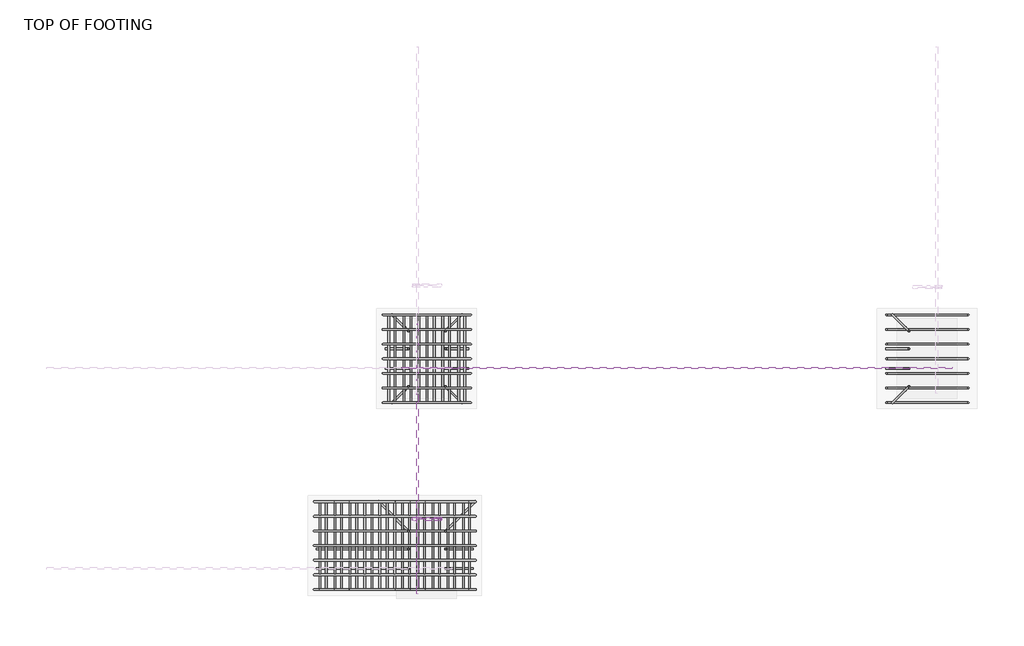
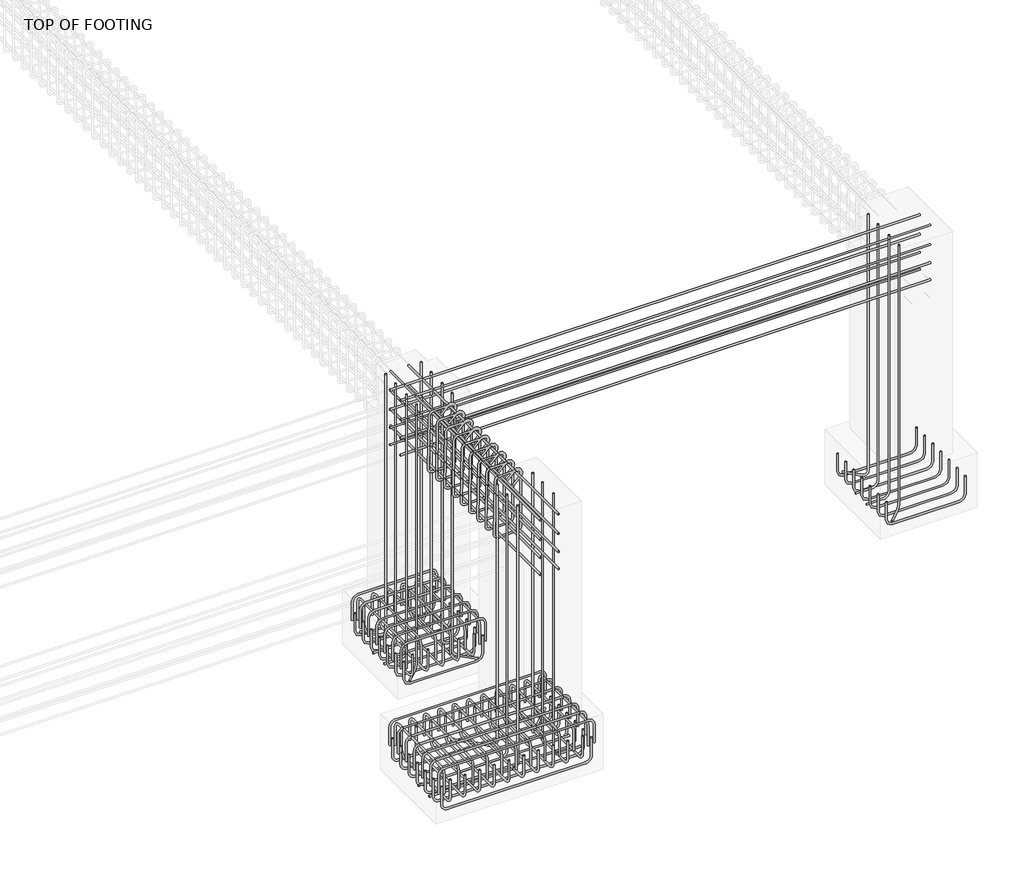
# One storey, part 3 of 8: 31 reinforcing bars.
"""IFC4 building model written with IfcOpenShell, lengths in millimetres."""

from ifc_helpers import new_model, si_unit, point, frame, origin, place, context, project, spatial, polyline, circle_curve, trimmed, segment, composite_curve, source, transform, mapped, element, save
from ifc_brep_helpers import swept_disk

model = new_model("IFC4")

# Units and contexts
model_context = context("Model", 3, world=origin())
ifc_project = project(units=[si_unit("LENGTHUNIT", "METRE", prefix="MILLI")], contexts=[model_context])

# Site, building, storey
site = spatial("IfcSite", under=ifc_project)
building = spatial("IfcBuilding", under=site)
storey = spatial("IfcBuildingStorey", under=building, Name="TOP OF FOOTING", Elevation=-1828.8)

# Reinforcing bars
placement = place(None, origin())
reinforcing_bar_shape = source(origin(), model_context, "Body", "SolidModel", [
    swept_disk(composite_curve([segment(polyline([(2354.4122182, -154.3579757, -2021.245224), (2354.4122182, -154.3579757, -2168.545224)]), True, "CONTINUOUS"), segment(trimmed(circle_curve(frame((2308.0622182, -154.3579757, -2168.545224), z_axis=(0.0, 1.0, 0.0), x_axis=(46.34999999999991, 0.0, 0.0)), 46.35), [point((2354.4122182, -154.3579757, -2168.545224))], [point((2308.0622182, -154.3579757, -2214.895224))], True, "CARTESIAN"), True, "CONTINUOUS"), segment(polyline([(2308.0622182, -154.3579757, -2214.895224), (1787.1241353, -154.3579757, -2214.895224)]), True, "CONTINUOUS"), segment(trimmed(circle_curve(frame((1787.1241353, -154.3579757, -2168.545224), z_axis=(0.0, 1.0, 0.0), x_axis=(0.0, 0.0, -46.34999999999991)), 46.35), [point((1787.1241353, -154.3579757, -2214.895224))], [point((1740.7741353, -154.3579757, -2168.545224))], True, "CARTESIAN"), True, "CONTINUOUS"), segment(polyline([(1740.7741353, -154.3579757, -2168.545224), (1740.7741353, -154.3579757, -2021.245224)]), True, "CONTINUOUS")], self_intersect=False), 6.35),
])
element("IfcReinforcingBar", 1, at=placement, inside=storey, context=model_context, shape_type="MappedRepresentation", body=[
    mapped(reinforcing_bar_shape, transform((0.0, 0.0, 0.0), x_axis=(1.0, 0.0, 0.0), y_axis=(0.0, 1.0, 0.0), z_axis=(0.0, 0.0, 1.0))),
    mapped(reinforcing_bar_shape, transform((0.0, -109.55, 0.0), x_axis=(1.0, 0.0, 0.0), y_axis=(0.0, 1.0, 0.0), z_axis=(0.0, 0.0, 1.0))),
    mapped(reinforcing_bar_shape, transform((0.0, -219.1, 0.0), x_axis=(1.0, 0.0, 0.0), y_axis=(0.0, 1.0, 0.0), z_axis=(0.0, 0.0, 1.0))),
    mapped(reinforcing_bar_shape, transform((0.0, -328.65, 0.0), x_axis=(1.0, 0.0, 0.0), y_axis=(0.0, 1.0, 0.0), z_axis=(0.0, 0.0, 1.0))),
    mapped(reinforcing_bar_shape, transform((0.0, -438.2, 0.0), x_axis=(1.0, 0.0, 0.0), y_axis=(0.0, 1.0, 0.0), z_axis=(0.0, 0.0, 1.0))),
    mapped(reinforcing_bar_shape, transform((0.0, -547.75, 0.0), x_axis=(1.0, 0.0, 0.0), y_axis=(0.0, 1.0, 0.0), z_axis=(0.0, 0.0, 1.0))),
    mapped(reinforcing_bar_shape, transform((0.0, -657.3, 0.0), x_axis=(1.0, 0.0, 0.0), y_axis=(0.0, 1.0, 0.0), z_axis=(0.0, 0.0, 1.0))),
])
reinforcing_bar_2_shape = source(origin(), model_context, "Body", "SolidModel", [
    swept_disk(composite_curve([segment(polyline([(-1395.5877818, -154.3579757, -2021.245224), (-1395.5877818, -154.3579757, -2168.545224)]), True, "CONTINUOUS"), segment(trimmed(circle_curve(frame((-1441.9377818, -154.3579757, -2168.545224), z_axis=(0.0, 1.0, 0.0), x_axis=(46.350000000000136, 0.0, 0.0)), 46.35), [point((-1395.5877818, -154.3579757, -2168.545224))], [point((-1441.9377818, -154.3579757, -2214.895224))], True, "CARTESIAN"), True, "CONTINUOUS"), segment(polyline([(-1441.9377818, -154.3579757, -2214.895224), (-1962.8758647, -154.3579757, -2214.895224)]), True, "CONTINUOUS"), segment(trimmed(circle_curve(frame((-1962.8758647, -154.3579757, -2168.545224), z_axis=(0.0, 1.0, 0.0), x_axis=(0.0, 0.0, -46.34999999999991)), 46.35), [point((-1962.8758647, -154.3579757, -2214.895224))], [point((-2009.2258647, -154.3579757, -2168.545224))], True, "CARTESIAN"), True, "CONTINUOUS"), segment(polyline([(-2009.2258647, -154.3579757, -2168.545224), (-2009.2258647, -154.3579757, -2021.245224)]), True, "CONTINUOUS")], self_intersect=False), 6.35),
])
element("IfcReinforcingBar", 2, at=placement, inside=storey, context=model_context, shape_type="MappedRepresentation", body=[
    mapped(reinforcing_bar_2_shape, transform((0.0, 0.0, 0.0), x_axis=(1.0, 0.0, 0.0), y_axis=(0.0, 1.0, 0.0), z_axis=(0.0, 0.0, 1.0))),
    mapped(reinforcing_bar_2_shape, transform((0.0, -109.55, 0.0), x_axis=(1.0, 0.0, 0.0), y_axis=(0.0, 1.0, 0.0), z_axis=(0.0, 0.0, 1.0))),
    mapped(reinforcing_bar_2_shape, transform((0.0, -219.1, 0.0), x_axis=(1.0, 0.0, 0.0), y_axis=(0.0, 1.0, 0.0), z_axis=(0.0, 0.0, 1.0))),
    mapped(reinforcing_bar_2_shape, transform((0.0, -328.65, 0.0), x_axis=(1.0, 0.0, 0.0), y_axis=(0.0, 1.0, 0.0), z_axis=(0.0, 0.0, 1.0))),
    mapped(reinforcing_bar_2_shape, transform((0.0, -438.2, 0.0), x_axis=(1.0, 0.0, 0.0), y_axis=(0.0, 1.0, 0.0), z_axis=(0.0, 0.0, 1.0))),
    mapped(reinforcing_bar_2_shape, transform((0.0, -547.75, 0.0), x_axis=(1.0, 0.0, 0.0), y_axis=(0.0, 1.0, 0.0), z_axis=(0.0, 0.0, 1.0))),
    mapped(reinforcing_bar_2_shape, transform((0.0, -657.3, 0.0), x_axis=(1.0, 0.0, 0.0), y_axis=(0.0, 1.0, 0.0), z_axis=(0.0, 0.0, 1.0))),
])
reinforcing_bar_3_shape = source(origin(), model_context, "Body", "SolidModel", [
    swept_disk(composite_curve([segment(polyline([(-2031.1461367, -154.3579757, -2068.8), (-2031.1461367, -154.3579757, -1921.5)]), True, "CONTINUOUS"), segment(trimmed(circle_curve(frame((-1984.7961367, -154.3579757, -1921.5), z_axis=(0.0, 1.0, 0.0), x_axis=(-46.34999999999991, 0.0, 0.0)), 46.35), [point((-2031.1461367, -154.3579757, -1921.5))], [point((-1984.7961367, -154.3579757, -1875.15))], True, "CARTESIAN"), True, "CONTINUOUS"), segment(polyline([(-1984.7961367, -154.3579757, -1875.15), (-1420.1961367, -154.3579757, -1875.15)]), True, "CONTINUOUS"), segment(trimmed(circle_curve(frame((-1420.1961367, -154.3579757, -1921.5), z_axis=(0.0, 1.0, 0.0), x_axis=(0.0, 0.0, 46.34999999999991)), 46.35), [point((-1420.1961367, -154.3579757, -1875.15))], [point((-1373.8461367, -154.3579757, -1921.5))], True, "CARTESIAN"), True, "CONTINUOUS"), segment(polyline([(-1373.8461367, -154.3579757, -1921.5), (-1373.8461367, -154.3579757, -2068.8)]), True, "CONTINUOUS")], self_intersect=False), 6.35),
])
element("IfcReinforcingBar", 3, at=placement, inside=storey, context=model_context, shape_type="MappedRepresentation", body=[
    mapped(reinforcing_bar_3_shape, transform((0.0, 0.0, 0.0), x_axis=(1.0, 0.0, 0.0), y_axis=(0.0, 1.0, 0.0), z_axis=(0.0, 0.0, 1.0))),
    mapped(reinforcing_bar_3_shape, transform((0.0, -109.55, 0.0), x_axis=(1.0, 0.0, 0.0), y_axis=(0.0, 1.0, 0.0), z_axis=(0.0, 0.0, 1.0))),
    mapped(reinforcing_bar_3_shape, transform((0.0, -219.1, 0.0), x_axis=(1.0, 0.0, 0.0), y_axis=(0.0, 1.0, 0.0), z_axis=(0.0, 0.0, 1.0))),
    mapped(reinforcing_bar_3_shape, transform((0.0, -328.65, 0.0), x_axis=(1.0, 0.0, 0.0), y_axis=(0.0, 1.0, 0.0), z_axis=(0.0, 0.0, 1.0))),
    mapped(reinforcing_bar_3_shape, transform((0.0, -438.2, 0.0), x_axis=(1.0, 0.0, 0.0), y_axis=(0.0, 1.0, 0.0), z_axis=(0.0, 0.0, 1.0))),
    mapped(reinforcing_bar_3_shape, transform((0.0, -547.75, 0.0), x_axis=(1.0, 0.0, 0.0), y_axis=(0.0, 1.0, 0.0), z_axis=(0.0, 0.0, 1.0))),
    mapped(reinforcing_bar_3_shape, transform((0.0, -657.3, 0.0), x_axis=(1.0, 0.0, 0.0), y_axis=(0.0, 1.0, 0.0), z_axis=(0.0, 0.0, 1.0))),
])
reinforcing_bar_4_shape = source(origin(), model_context, "Body", "SolidModel", [
    swept_disk(composite_curve([segment(polyline([(-1419.0253093, -154.3579757, -2080.9203068), (-1419.0253093, -154.3579757, -1933.6203068)]), True, "CONTINUOUS"), segment(trimmed(circle_curve(frame((-1419.0253093, -200.7079757, -1933.6203068), z_axis=(1.0, 0.0, 0.0), x_axis=(0.0, 46.349999999999994, 0.0)), 46.35), [point((-1419.0253093, -154.3579757, -1933.6203068))], [point((-1419.0253093, -200.7079757, -1887.2703068))], True, "CARTESIAN"), True, "CONTINUOUS"), segment(polyline([(-1419.0253093, -200.7079757, -1887.2703068), (-1419.0253093, -765.3079757, -1887.2703068)]), True, "CONTINUOUS"), segment(trimmed(circle_curve(frame((-1419.0253093, -765.3079757, -1933.6203068), z_axis=(1.0, 0.0, 0.0), x_axis=(0.0, 0.0, 46.34999999999991)), 46.35), [point((-1419.0253093, -765.3079757, -1887.2703068))], [point((-1419.0253093, -811.6579757, -1933.6203068))], True, "CARTESIAN"), True, "CONTINUOUS"), segment(polyline([(-1419.0253093, -811.6579757, -1933.6203068), (-1419.0253093, -811.6579757, -2080.9203068)]), True, "CONTINUOUS")], self_intersect=False), 6.35),
])
element("IfcReinforcingBar", 4, at=placement, inside=storey, context=model_context, shape_type="MappedRepresentation", body=[
    mapped(reinforcing_bar_4_shape, transform((0.0, 0.0, 0.0), x_axis=(1.0, 0.0, 0.0), y_axis=(0.0, 1.0, 0.0), z_axis=(0.0, 0.0, 1.0))),
    mapped(reinforcing_bar_4_shape, transform((-113.9683653, 0.0, 0.0), x_axis=(1.0, 0.0, 0.0), y_axis=(0.0, 1.0, 0.0), z_axis=(0.0, 0.0, 1.0))),
    mapped(reinforcing_bar_4_shape, transform((-227.9367307, 0.0, 0.0), x_axis=(1.0, 0.0, 0.0), y_axis=(0.0, 1.0, 0.0), z_axis=(0.0, 0.0, 1.0))),
    mapped(reinforcing_bar_4_shape, transform((-341.905096, 0.0, 0.0), x_axis=(1.0, 0.0, 0.0), y_axis=(0.0, 1.0, 0.0), z_axis=(0.0, 0.0, 1.0))),
    mapped(reinforcing_bar_4_shape, transform((-455.8734613, 0.0, 0.0), x_axis=(1.0, 0.0, 0.0), y_axis=(0.0, 1.0, 0.0), z_axis=(0.0, 0.0, 1.0))),
    mapped(reinforcing_bar_4_shape, transform((-569.8418267, 0.0, 0.0), x_axis=(1.0, 0.0, 0.0), y_axis=(0.0, 1.0, 0.0), z_axis=(0.0, 0.0, 1.0))),
])
reinforcing_bar_5_shape = source(origin(), model_context, "Body", "SolidModel", [
    swept_disk(composite_curve([segment(polyline([(-1941.3656272, -154.3579757, -1984.9681267), (-1941.3656272, -154.3579757, -2132.2681267)]), True, "CONTINUOUS"), segment(trimmed(circle_curve(frame((-1941.3656272, -200.7079757, -2132.2681267), z_axis=(-1.0, 0.0, 0.0), x_axis=(0.0, 46.349999999999994, 0.0)), 46.35), [point((-1941.3656272, -154.3579757, -2132.2681267))], [point((-1941.3656272, -200.7079757, -2178.6181267))], True, "CARTESIAN"), True, "CONTINUOUS"), segment(polyline([(-1941.3656272, -200.7079757, -2178.6181267), (-1941.3656272, -765.3079757, -2178.6181267)]), True, "CONTINUOUS"), segment(trimmed(circle_curve(frame((-1941.3656272, -765.3079757, -2132.2681267), z_axis=(-1.0, 0.0, 0.0), x_axis=(0.0, 0.0, -46.350000000000364)), 46.35), [point((-1941.3656272, -765.3079757, -2178.6181267))], [point((-1941.3656272, -811.6579757, -2132.2681267))], True, "CARTESIAN"), True, "CONTINUOUS"), segment(polyline([(-1941.3656272, -811.6579757, -2132.2681267), (-1941.3656272, -811.6579757, -1984.9681267)]), True, "CONTINUOUS")], self_intersect=False), 6.35),
])
element("IfcReinforcingBar", 5, at=placement, inside=storey, context=model_context, shape_type="MappedRepresentation", body=[
    mapped(reinforcing_bar_5_shape, transform((0.0, 0.0, 0.0), x_axis=(1.0, 0.0, 0.0), y_axis=(0.0, 1.0, 0.0), z_axis=(0.0, 0.0, 1.0))),
    mapped(reinforcing_bar_5_shape, transform((119.2770606, 0.0, 0.0), x_axis=(1.0, 0.0, 0.0), y_axis=(0.0, 1.0, 0.0), z_axis=(0.0, 0.0, 1.0))),
    mapped(reinforcing_bar_5_shape, transform((238.5541211, 0.0, 0.0), x_axis=(1.0, 0.0, 0.0), y_axis=(0.0, 1.0, 0.0), z_axis=(0.0, 0.0, 1.0))),
    mapped(reinforcing_bar_5_shape, transform((357.8311817, 0.0, 0.0), x_axis=(1.0, 0.0, 0.0), y_axis=(0.0, 1.0, 0.0), z_axis=(0.0, 0.0, 1.0))),
    mapped(reinforcing_bar_5_shape, transform((477.1082423, 0.0, 0.0), x_axis=(1.0, 0.0, 0.0), y_axis=(0.0, 1.0, 0.0), z_axis=(0.0, 0.0, 1.0))),
])
reinforcing_bar_6_shape = source(origin(), model_context, "Body", "SolidModel", [
    swept_disk(composite_curve([segment(polyline([(-1360.5877818, -1554.3579757, -2021.245224), (-1360.5877818, -1554.3579757, -2168.545224)]), True, "CONTINUOUS"), segment(trimmed(circle_curve(frame((-1406.9377818, -1554.3579757, -2168.545224), z_axis=(0.0, 1.0, 0.0), x_axis=(46.350000000000136, 0.0, 0.0)), 46.35), [point((-1360.5877818, -1554.3579757, -2168.545224))], [point((-1406.9377818, -1554.3579757, -2214.895224))], True, "CARTESIAN"), True, "CONTINUOUS"), segment(polyline([(-1406.9377818, -1554.3579757, -2214.895224), (-2477.8758647, -1554.3579757, -2214.895224)]), True, "CONTINUOUS"), segment(trimmed(circle_curve(frame((-2477.8758647, -1554.3579757, -2168.545224), z_axis=(0.0, 1.0, 0.0), x_axis=(0.0, 0.0, -46.34999999999991)), 46.35), [point((-2477.8758647, -1554.3579757, -2214.895224))], [point((-2524.2258647, -1554.3579757, -2168.545224))], True, "CARTESIAN"), True, "CONTINUOUS"), segment(polyline([(-2524.2258647, -1554.3579757, -2168.545224), (-2524.2258647, -1554.3579757, -2021.245224)]), True, "CONTINUOUS")], self_intersect=False), 6.35),
])
element("IfcReinforcingBar", 6, at=placement, inside=storey, context=model_context, shape_type="MappedRepresentation", body=[
    mapped(reinforcing_bar_6_shape, transform((0.0, 0.0, 0.0), x_axis=(1.0, 0.0, 0.0), y_axis=(0.0, 1.0, 0.0), z_axis=(0.0, 0.0, 1.0))),
    mapped(reinforcing_bar_6_shape, transform((0.0, -109.55, 0.0), x_axis=(1.0, 0.0, 0.0), y_axis=(0.0, 1.0, 0.0), z_axis=(0.0, 0.0, 1.0))),
    mapped(reinforcing_bar_6_shape, transform((0.0, -219.1, 0.0), x_axis=(1.0, 0.0, 0.0), y_axis=(0.0, 1.0, 0.0), z_axis=(0.0, 0.0, 1.0))),
    mapped(reinforcing_bar_6_shape, transform((0.0, -328.65, 0.0), x_axis=(1.0, 0.0, 0.0), y_axis=(0.0, 1.0, 0.0), z_axis=(0.0, 0.0, 1.0))),
    mapped(reinforcing_bar_6_shape, transform((0.0, -438.2, 0.0), x_axis=(1.0, 0.0, 0.0), y_axis=(0.0, 1.0, 0.0), z_axis=(0.0, 0.0, 1.0))),
    mapped(reinforcing_bar_6_shape, transform((0.0, -547.75, 0.0), x_axis=(1.0, 0.0, 0.0), y_axis=(0.0, 1.0, 0.0), z_axis=(0.0, 0.0, 1.0))),
    mapped(reinforcing_bar_6_shape, transform((0.0, -657.3, 0.0), x_axis=(1.0, 0.0, 0.0), y_axis=(0.0, 1.0, 0.0), z_axis=(0.0, 0.0, 1.0))),
])
reinforcing_bar_7_shape = source(origin(), model_context, "Body", "SolidModel", [
    swept_disk(composite_curve([segment(polyline([(-2546.1461367, -1554.3579757, -2068.8), (-2546.1461367, -1554.3579757, -1921.5)]), True, "CONTINUOUS"), segment(trimmed(circle_curve(frame((-2499.7961367, -1554.3579757, -1921.5), z_axis=(0.0, 1.0, 0.0), x_axis=(-46.350000000000364, 0.0, 0.0)), 46.35), [point((-2546.1461367, -1554.3579757, -1921.5))], [point((-2499.7961367, -1554.3579757, -1875.15))], True, "CARTESIAN"), True, "CONTINUOUS"), segment(polyline([(-2499.7961367, -1554.3579757, -1875.15), (-1385.1961367, -1554.3579757, -1875.15)]), True, "CONTINUOUS"), segment(trimmed(circle_curve(frame((-1385.1961367, -1554.3579757, -1921.5), z_axis=(0.0, 1.0, 0.0), x_axis=(0.0, 0.0, 46.34999999999991)), 46.35), [point((-1385.1961367, -1554.3579757, -1875.15))], [point((-1338.8461367, -1554.3579757, -1921.5))], True, "CARTESIAN"), True, "CONTINUOUS"), segment(polyline([(-1338.8461367, -1554.3579757, -1921.5), (-1338.8461367, -1554.3579757, -2068.8)]), True, "CONTINUOUS")], self_intersect=False), 6.35),
])
element("IfcReinforcingBar", 7, at=placement, inside=storey, context=model_context, shape_type="MappedRepresentation", body=[
    mapped(reinforcing_bar_7_shape, transform((0.0, 0.0, 0.0), x_axis=(1.0, 0.0, 0.0), y_axis=(0.0, 1.0, 0.0), z_axis=(0.0, 0.0, 1.0))),
    mapped(reinforcing_bar_7_shape, transform((0.0, -109.55, 0.0), x_axis=(1.0, 0.0, 0.0), y_axis=(0.0, 1.0, 0.0), z_axis=(0.0, 0.0, 1.0))),
    mapped(reinforcing_bar_7_shape, transform((0.0, -219.1, 0.0), x_axis=(1.0, 0.0, 0.0), y_axis=(0.0, 1.0, 0.0), z_axis=(0.0, 0.0, 1.0))),
    mapped(reinforcing_bar_7_shape, transform((0.0, -328.65, 0.0), x_axis=(1.0, 0.0, 0.0), y_axis=(0.0, 1.0, 0.0), z_axis=(0.0, 0.0, 1.0))),
    mapped(reinforcing_bar_7_shape, transform((0.0, -438.2, 0.0), x_axis=(1.0, 0.0, 0.0), y_axis=(0.0, 1.0, 0.0), z_axis=(0.0, 0.0, 1.0))),
    mapped(reinforcing_bar_7_shape, transform((0.0, -547.75, 0.0), x_axis=(1.0, 0.0, 0.0), y_axis=(0.0, 1.0, 0.0), z_axis=(0.0, 0.0, 1.0))),
    mapped(reinforcing_bar_7_shape, transform((0.0, -657.3, 0.0), x_axis=(1.0, 0.0, 0.0), y_axis=(0.0, 1.0, 0.0), z_axis=(0.0, 0.0, 1.0))),
])
reinforcing_bar_8_shape = source(origin(), model_context, "Body", "SolidModel", [
    swept_disk(composite_curve([segment(polyline([(-1384.0253093, -1554.3579757, -2080.9203068), (-1384.0253093, -1554.3579757, -1933.6203068)]), True, "CONTINUOUS"), segment(trimmed(circle_curve(frame((-1384.0253093, -1600.7079757, -1933.6203068), z_axis=(1.0, 0.0, 0.0), x_axis=(0.0, 46.34999999999991, 0.0)), 46.35), [point((-1384.0253093, -1554.3579757, -1933.6203068))], [point((-1384.0253093, -1600.7079757, -1887.2703068))], True, "CARTESIAN"), True, "CONTINUOUS"), segment(polyline([(-1384.0253093, -1600.7079757, -1887.2703068), (-1384.0253093, -2165.3079757, -1887.2703068)]), True, "CONTINUOUS"), segment(trimmed(circle_curve(frame((-1384.0253093, -2165.3079757, -1933.6203068), z_axis=(1.0, 0.0, 0.0), x_axis=(0.0, 0.0, 46.34999999999991)), 46.35), [point((-1384.0253093, -2165.3079757, -1887.2703068))], [point((-1384.0253093, -2211.6579757, -1933.6203068))], True, "CARTESIAN"), True, "CONTINUOUS"), segment(polyline([(-1384.0253093, -2211.6579757, -1933.6203068), (-1384.0253093, -2211.6579757, -2080.9203068)]), True, "CONTINUOUS")], self_intersect=False), 6.35),
])
element("IfcReinforcingBar", 8, at=placement, inside=storey, context=model_context, shape_type="MappedRepresentation", body=[
    mapped(reinforcing_bar_8_shape, transform((0.0, 0.0, 0.0), x_axis=(1.0, 0.0, 0.0), y_axis=(0.0, 1.0, 0.0), z_axis=(0.0, 0.0, 1.0))),
    mapped(reinforcing_bar_8_shape, transform((-111.9841827, 0.0, 0.0), x_axis=(1.0, 0.0, 0.0), y_axis=(0.0, 1.0, 0.0), z_axis=(0.0, 0.0, 1.0))),
    mapped(reinforcing_bar_8_shape, transform((-223.9683653, 0.0, 0.0), x_axis=(1.0, 0.0, 0.0), y_axis=(0.0, 1.0, 0.0), z_axis=(0.0, 0.0, 1.0))),
    mapped(reinforcing_bar_8_shape, transform((-335.952548, 0.0, 0.0), x_axis=(1.0, 0.0, 0.0), y_axis=(0.0, 1.0, 0.0), z_axis=(0.0, 0.0, 1.0))),
    mapped(reinforcing_bar_8_shape, transform((-447.9367307, 0.0, 0.0), x_axis=(1.0, 0.0, 0.0), y_axis=(0.0, 1.0, 0.0), z_axis=(0.0, 0.0, 1.0))),
    mapped(reinforcing_bar_8_shape, transform((-559.9209133, 0.0, 0.0), x_axis=(1.0, 0.0, 0.0), y_axis=(0.0, 1.0, 0.0), z_axis=(0.0, 0.0, 1.0))),
    mapped(reinforcing_bar_8_shape, transform((-671.905096, 0.0, 0.0), x_axis=(1.0, 0.0, 0.0), y_axis=(0.0, 1.0, 0.0), z_axis=(0.0, 0.0, 1.0))),
    mapped(reinforcing_bar_8_shape, transform((-783.8892787, 0.0, 0.0), x_axis=(1.0, 0.0, 0.0), y_axis=(0.0, 1.0, 0.0), z_axis=(0.0, 0.0, 1.0))),
    mapped(reinforcing_bar_8_shape, transform((-895.8734613, 0.0, 0.0), x_axis=(1.0, 0.0, 0.0), y_axis=(0.0, 1.0, 0.0), z_axis=(0.0, 0.0, 1.0))),
    mapped(reinforcing_bar_8_shape, transform((-1007.857644, 0.0, 0.0), x_axis=(1.0, 0.0, 0.0), y_axis=(0.0, 1.0, 0.0), z_axis=(0.0, 0.0, 1.0))),
    mapped(reinforcing_bar_8_shape, transform((-1119.8418267, 0.0, 0.0), x_axis=(1.0, 0.0, 0.0), y_axis=(0.0, 1.0, 0.0), z_axis=(0.0, 0.0, 1.0))),
])
reinforcing_bar_9_shape = source(origin(), model_context, "Body", "SolidModel", [
    swept_disk(composite_curve([segment(polyline([(-2456.3656272, -1554.3579757, -1984.9681267), (-2456.3656272, -1554.3579757, -2132.2681267)]), True, "CONTINUOUS"), segment(trimmed(circle_curve(frame((-2456.3656272, -1600.7079757, -2132.2681267), z_axis=(-1.0, 0.0, 0.0), x_axis=(0.0, 46.34999999999991, 0.0)), 46.35), [point((-2456.3656272, -1554.3579757, -2132.2681267))], [point((-2456.3656272, -1600.7079757, -2178.6181267))], True, "CARTESIAN"), True, "CONTINUOUS"), segment(polyline([(-2456.3656272, -1600.7079757, -2178.6181267), (-2456.3656272, -2165.3079757, -2178.6181267)]), True, "CONTINUOUS"), segment(trimmed(circle_curve(frame((-2456.3656272, -2165.3079757, -2132.2681267), z_axis=(-1.0, 0.0, 0.0), x_axis=(0.0, 0.0, -46.350000000000364)), 46.35), [point((-2456.3656272, -2165.3079757, -2178.6181267))], [point((-2456.3656272, -2211.6579757, -2132.2681267))], True, "CARTESIAN"), True, "CONTINUOUS"), segment(polyline([(-2456.3656272, -2211.6579757, -2132.2681267), (-2456.3656272, -2211.6579757, -1984.9681267)]), True, "CONTINUOUS")], self_intersect=False), 6.35),
])
element("IfcReinforcingBar", 9, at=placement, inside=storey, context=model_context, shape_type="MappedRepresentation", body=[
    mapped(reinforcing_bar_9_shape, transform((0.0, 0.0, 0.0), x_axis=(1.0, 0.0, 0.0), y_axis=(0.0, 1.0, 0.0), z_axis=(0.0, 0.0, 1.0))),
    mapped(reinforcing_bar_9_shape, transform((114.123138, 0.0, 0.0), x_axis=(1.0, 0.0, 0.0), y_axis=(0.0, 1.0, 0.0), z_axis=(0.0, 0.0, 1.0))),
    mapped(reinforcing_bar_9_shape, transform((228.2462761, 0.0, 0.0), x_axis=(1.0, 0.0, 0.0), y_axis=(0.0, 1.0, 0.0), z_axis=(0.0, 0.0, 1.0))),
    mapped(reinforcing_bar_9_shape, transform((342.3694141, 0.0, 0.0), x_axis=(1.0, 0.0, 0.0), y_axis=(0.0, 1.0, 0.0), z_axis=(0.0, 0.0, 1.0))),
    mapped(reinforcing_bar_9_shape, transform((456.4925521, 0.0, 0.0), x_axis=(1.0, 0.0, 0.0), y_axis=(0.0, 1.0, 0.0), z_axis=(0.0, 0.0, 1.0))),
    mapped(reinforcing_bar_9_shape, transform((570.6156901, 0.0, 0.0), x_axis=(1.0, 0.0, 0.0), y_axis=(0.0, 1.0, 0.0), z_axis=(0.0, 0.0, 1.0))),
    mapped(reinforcing_bar_9_shape, transform((684.7388282, 0.0, 0.0), x_axis=(1.0, 0.0, 0.0), y_axis=(0.0, 1.0, 0.0), z_axis=(0.0, 0.0, 1.0))),
    mapped(reinforcing_bar_9_shape, transform((798.8619662, 0.0, 0.0), x_axis=(1.0, 0.0, 0.0), y_axis=(0.0, 1.0, 0.0), z_axis=(0.0, 0.0, 1.0))),
    mapped(reinforcing_bar_9_shape, transform((912.9851042, 0.0, 0.0), x_axis=(1.0, 0.0, 0.0), y_axis=(0.0, 1.0, 0.0), z_axis=(0.0, 0.0, 1.0))),
    mapped(reinforcing_bar_9_shape, transform((1027.1082423, 0.0, 0.0), x_axis=(1.0, 0.0, 0.0), y_axis=(0.0, 1.0, 0.0), z_axis=(0.0, 0.0, 1.0))),
])
reinforcing_bar_10_shape = source(origin(), model_context, "Body", "SolidModel", [
    swept_disk(composite_curve([segment(polyline([(1734.5561653, -407.8655692, -2192.6897268), (1862.8848277, -407.8655692, -2192.6897268)]), True, "CONTINUOUS"), segment(trimmed(circle_curve(frame((1862.8848277, -407.8655692, -2146.3397268), z_axis=(0.0, -1.0, 0.0), x_axis=(0.0, 0.0, -46.34999999999991)), 46.35), [point((1862.8848277, -407.8655692, -2192.6897268))], [point((1909.2348277, -407.8655692, -2146.3397268))], True, "CARTESIAN"), True, "CONTINUOUS"), segment(polyline([(1909.2348277, -407.8655692, -2146.3397268), (1909.2348277, -407.8655692, -40.0)]), True, "CONTINUOUS")], self_intersect=False), 6.35),
])
element("IfcReinforcingBar", 10, at=placement, inside=storey, context=model_context, shape_type="MappedRepresentation", body=[
    mapped(reinforcing_bar_10_shape, transform((0.0, 0.0, 0.0), x_axis=(1.0, 0.0, 0.0), y_axis=(0.0, 1.0, 0.0), z_axis=(0.0, 0.0, 1.0))),
    mapped(reinforcing_bar_10_shape, transform((0.0, -147.7903727, 0.0), x_axis=(1.0, 0.0, 0.0), y_axis=(0.0, 1.0, 0.0), z_axis=(0.0, 0.0, 1.0))),
])
element("IfcReinforcingBar", 11, at=placement, inside=storey, context=model_context, shape_type="SolidModel", body=[
    swept_disk(composite_curve([segment(polyline([(1781.9855998, -817.3699065, -2192.6897268), (1876.4604283, -722.8950779, -2192.6897268)]), True, "CONTINUOUS"), segment(trimmed(circle_curve(frame((1876.4604283, -722.8950779, -2146.3397268), z_axis=(0.7071067811865476, -0.7071067811865475, 0.0), x_axis=(0.0, 0.0, -46.34999999999991)), 46.35), [point((1876.4604283, -722.8950779, -2192.6897268))], [point((1909.2348277, -690.1206786, -2146.3397268))], True, "CARTESIAN"), True, "CONTINUOUS"), segment(polyline([(1909.2348277, -690.1206786, -2146.3397268), (1909.2348277, -690.1206786, -40.0)]), True, "CONTINUOUS")], self_intersect=False), 6.35),
])
element("IfcReinforcingBar", 12, at=placement, inside=storey, context=model_context, shape_type="SolidModel", body=[
    swept_disk(composite_curve([segment(polyline([(1781.9855998, -148.646045, -2192.6897268), (1876.4604283, -243.1208736, -2192.6897268)]), True, "CONTINUOUS"), segment(trimmed(circle_curve(frame((1876.4604283, -243.1208736, -2146.3397268), z_axis=(-0.7071067811865389, -0.7071067811865561, 0.0), x_axis=(0.0, 0.0, -46.34999999999991)), 46.35), [point((1876.4604283, -243.1208736, -2192.6897268))], [point((1909.2348277, -275.8952729, -2146.3397268))], True, "CARTESIAN"), True, "CONTINUOUS"), segment(polyline([(1909.2348277, -275.8952729, -2146.3397268), (1909.2348277, -275.8952729, -40.0)]), True, "CONTINUOUS")], self_intersect=False), 6.35),
])
reinforcing_bar_11_shape = source(origin(), model_context, "Body", "SolidModel", [
    swept_disk(composite_curve([segment(polyline([(-2015.4438347, -407.8655692, -2192.6897268), (-1887.1151723, -407.8655692, -2192.6897268)]), True, "CONTINUOUS"), segment(trimmed(circle_curve(frame((-1887.1151723, -407.8655692, -2146.3397268), z_axis=(0.0, -1.0, 0.0), x_axis=(0.0, 0.0, -46.34999999999991)), 46.35), [point((-1887.1151723, -407.8655692, -2192.6897268))], [point((-1840.7651723, -407.8655692, -2146.3397268))], True, "CARTESIAN"), True, "CONTINUOUS"), segment(polyline([(-1840.7651723, -407.8655692, -2146.3397268), (-1840.7651723, -407.8655692, -40.0)]), True, "CONTINUOUS")], self_intersect=False), 6.35),
])
element("IfcReinforcingBar", 13, at=placement, inside=storey, context=model_context, shape_type="MappedRepresentation", body=[
    mapped(reinforcing_bar_11_shape, transform((0.0, 0.0, 0.0), x_axis=(1.0, 0.0, 0.0), y_axis=(0.0, 1.0, 0.0), z_axis=(0.0, 0.0, 1.0))),
    mapped(reinforcing_bar_11_shape, transform((0.0, -147.7903727, 0.0), x_axis=(1.0, 0.0, 0.0), y_axis=(0.0, 1.0, 0.0), z_axis=(0.0, 0.0, 1.0))),
])
element("IfcReinforcingBar", 14, at=placement, inside=storey, context=model_context, shape_type="SolidModel", body=[
    swept_disk(composite_curve([segment(polyline([(-1968.0144002, -817.3699065, -2192.6897268), (-1873.5395717, -722.8950779, -2192.6897268)]), True, "CONTINUOUS"), segment(trimmed(circle_curve(frame((-1873.5395717, -722.8950779, -2146.3397268), z_axis=(0.7071067811865476, -0.7071067811865475, 0.0), x_axis=(0.0, 0.0, -46.34999999999991)), 46.35), [point((-1873.5395717, -722.8950779, -2192.6897268))], [point((-1840.7651723, -690.1206786, -2146.3397268))], True, "CARTESIAN"), True, "CONTINUOUS"), segment(polyline([(-1840.7651723, -690.1206786, -2146.3397268), (-1840.7651723, -690.1206786, -40.0)]), True, "CONTINUOUS")], self_intersect=False), 6.35),
])
element("IfcReinforcingBar", 15, at=placement, inside=storey, context=model_context, shape_type="SolidModel", body=[
    swept_disk(composite_curve([segment(polyline([(-1436.9778732, -817.3699065, -2192.6897268), (-1531.4527018, -722.8950779, -2192.6897268)]), True, "CONTINUOUS"), segment(trimmed(circle_curve(frame((-1531.4527018, -722.8950779, -2146.3397268), z_axis=(0.7071067811865753, 0.7071067811865197, 0.0), x_axis=(0.0, 0.0, -46.34999999999991)), 46.35), [point((-1531.4527018, -722.8950779, -2192.6897268))], [point((-1564.2271011, -690.1206786, -2146.3397268))], True, "CARTESIAN"), True, "CONTINUOUS"), segment(polyline([(-1564.2271011, -690.1206786, -2146.3397268), (-1564.2271011, -690.1206786, -40.0)]), True, "CONTINUOUS")], self_intersect=False), 6.35),
])
element("IfcReinforcingBar", 16, at=placement, inside=storey, context=model_context, shape_type="SolidModel", body=[
    swept_disk(composite_curve([segment(polyline([(-1968.0144002, -148.646045, -2192.6897268), (-1873.5395717, -243.1208736, -2192.6897268)]), True, "CONTINUOUS"), segment(trimmed(circle_curve(frame((-1873.5395717, -243.1208736, -2146.3397268), z_axis=(-0.7071067811865389, -0.7071067811865561, 0.0), x_axis=(0.0, 0.0, -46.34999999999991)), 46.35), [point((-1873.5395717, -243.1208736, -2192.6897268))], [point((-1840.7651723, -275.8952729, -2146.3397268))], True, "CARTESIAN"), True, "CONTINUOUS"), segment(polyline([(-1840.7651723, -275.8952729, -2146.3397268), (-1840.7651723, -275.8952729, -40.0)]), True, "CONTINUOUS")], self_intersect=False), 6.35),
])
element("IfcReinforcingBar", 17, at=placement, inside=storey, context=model_context, shape_type="SolidModel", body=[
    swept_disk(composite_curve([segment(polyline([(-1436.9778732, -148.646045, -2192.6897268), (-1531.4527018, -243.1208736, -2192.6897268)]), True, "CONTINUOUS"), segment(trimmed(circle_curve(frame((-1531.4527018, -243.1208736, -2146.3397268), z_axis=(-0.707106781186584, 0.707106781186511, 0.0), x_axis=(0.0, 0.0, -46.34999999999991)), 46.35), [point((-1531.4527018, -243.1208736, -2192.6897268))], [point((-1564.2271011, -275.8952729, -2146.3397268))], True, "CARTESIAN"), True, "CONTINUOUS"), segment(polyline([(-1564.2271011, -275.8952729, -2146.3397268), (-1564.2271011, -275.8952729, -40.0)]), True, "CONTINUOUS")], self_intersect=False), 6.35),
])
reinforcing_bar_12_shape = source(origin(), model_context, "Body", "SolidModel", [
    swept_disk(composite_curve([segment(polyline([(-1389.5484388, -407.8655692, -2192.6897268), (-1517.8771011, -407.8655692, -2192.6897268)]), True, "CONTINUOUS"), segment(trimmed(circle_curve(frame((-1517.8771011, -407.8655692, -2146.3397268), z_axis=(0.0, 1.0, 0.0), x_axis=(0.0, 0.0, -46.34999999999991)), 46.35), [point((-1517.8771011, -407.8655692, -2192.6897268))], [point((-1564.2271011, -407.8655692, -2146.3397268))], True, "CARTESIAN"), True, "CONTINUOUS"), segment(polyline([(-1564.2271011, -407.8655692, -2146.3397268), (-1564.2271011, -407.8655692, -40.0)]), True, "CONTINUOUS")], self_intersect=False), 6.35),
])
element("IfcReinforcingBar", 18, at=placement, inside=storey, context=model_context, shape_type="MappedRepresentation", body=[
    mapped(reinforcing_bar_12_shape, transform((0.0, 0.0, 0.0), x_axis=(1.0, 0.0, 0.0), y_axis=(0.0, 1.0, 0.0), z_axis=(0.0, 0.0, 1.0))),
    mapped(reinforcing_bar_12_shape, transform((0.0, -147.7903727, 0.0), x_axis=(1.0, 0.0, 0.0), y_axis=(0.0, 1.0, 0.0), z_axis=(0.0, 0.0, 1.0))),
])
reinforcing_bar_13_shape = source(origin(), model_context, "Body", "SolidModel", [
    swept_disk(composite_curve([segment(polyline([(-2530.4438347, -1907.8655692, -2192.6897268), (-1887.1151723, -1907.8655692, -2192.6897268)]), True, "CONTINUOUS"), segment(trimmed(circle_curve(frame((-1887.1151723, -1907.8655692, -2146.3397268), z_axis=(0.0, -1.0, 0.0), x_axis=(0.0, 0.0, -46.34999999999991)), 46.35), [point((-1887.1151723, -1907.8655692, -2192.6897268))], [point((-1840.7651723, -1907.8655692, -2146.3397268))], True, "CARTESIAN"), True, "CONTINUOUS"), segment(polyline([(-1840.7651723, -1907.8655692, -2146.3397268), (-1840.7651723, -1907.8655692, -40.0)]), True, "CONTINUOUS")], self_intersect=False), 6.35),
])
element("IfcReinforcingBar", 19, at=placement, inside=storey, context=model_context, shape_type="MappedRepresentation", body=[
    mapped(reinforcing_bar_13_shape, transform((0.0, 0.0, 0.0), x_axis=(1.0, 0.0, 0.0), y_axis=(0.0, 1.0, 0.0), z_axis=(0.0, 0.0, 1.0))),
    mapped(reinforcing_bar_13_shape, transform((0.0, -147.7903727, 0.0), x_axis=(1.0, 0.0, 0.0), y_axis=(0.0, 1.0, 0.0), z_axis=(0.0, 0.0, 1.0))),
])
element("IfcReinforcingBar", 20, at=placement, inside=storey, context=model_context, shape_type="SolidModel", body=[
    swept_disk(composite_curve([segment(polyline([(-2068.0144002, -1548.646045, -2192.6897268), (-1873.5395717, -1743.1208736, -2192.6897268)]), True, "CONTINUOUS"), segment(trimmed(circle_curve(frame((-1873.5395717, -1743.1208736, -2146.3397268), z_axis=(-0.7071067811865389, -0.7071067811865561, 0.0), x_axis=(0.0, 0.0, -46.34999999999991)), 46.35), [point((-1873.5395717, -1743.1208736, -2192.6897268))], [point((-1840.7651723, -1775.8952729, -2146.3397268))], True, "CARTESIAN"), True, "CONTINUOUS"), segment(polyline([(-1840.7651723, -1775.8952729, -2146.3397268), (-1840.7651723, -1775.8952729, -40.0)]), True, "CONTINUOUS")], self_intersect=False), 6.35),
])
element("IfcReinforcingBar", 21, at=placement, inside=storey, context=model_context, shape_type="SolidModel", body=[
    swept_disk(composite_curve([segment(polyline([(-1336.9778732, -1548.646045, -2192.6897268), (-1531.4527018, -1743.1208736, -2192.6897268)]), True, "CONTINUOUS"), segment(trimmed(circle_curve(frame((-1531.4527018, -1743.1208736, -2146.3397268), z_axis=(-0.707106781186584, 0.707106781186511, 0.0), x_axis=(0.0, 0.0, -46.34999999999991)), 46.35), [point((-1531.4527018, -1743.1208736, -2192.6897268))], [point((-1564.2271011, -1775.8952729, -2146.3397268))], True, "CARTESIAN"), True, "CONTINUOUS"), segment(polyline([(-1564.2271011, -1775.8952729, -2146.3397268), (-1564.2271011, -1775.8952729, -40.0)]), True, "CONTINUOUS")], self_intersect=False), 6.35),
])
reinforcing_bar_14_shape = source(origin(), model_context, "Body", "SolidModel", [
    swept_disk(composite_curve([segment(polyline([(-1354.5484388, -1907.8655692, -2192.6897268), (-1517.8771011, -1907.8655692, -2192.6897268)]), True, "CONTINUOUS"), segment(trimmed(circle_curve(frame((-1517.8771011, -1907.8655692, -2146.3397268), z_axis=(0.0, 1.0, 0.0), x_axis=(0.0, 0.0, -46.34999999999991)), 46.35), [point((-1517.8771011, -1907.8655692, -2192.6897268))], [point((-1564.2271011, -1907.8655692, -2146.3397268))], True, "CARTESIAN"), True, "CONTINUOUS"), segment(polyline([(-1564.2271011, -1907.8655692, -2146.3397268), (-1564.2271011, -1907.8655692, -40.0)]), True, "CONTINUOUS")], self_intersect=False), 6.35),
])
element("IfcReinforcingBar", 22, at=placement, inside=storey, context=model_context, shape_type="MappedRepresentation", body=[
    mapped(reinforcing_bar_14_shape, transform((0.0, 0.0, 0.0), x_axis=(1.0, 0.0, 0.0), y_axis=(0.0, 1.0, 0.0), z_axis=(0.0, 0.0, 1.0))),
    mapped(reinforcing_bar_14_shape, transform((0.0, -147.7903727, 0.0), x_axis=(1.0, 0.0, 0.0), y_axis=(0.0, 1.0, 0.0), z_axis=(0.0, 0.0, 1.0))),
])
reinforcing_bar_15_shape = source(origin(), model_context, "Body", "SolidModel", [
    swept_disk(composite_curve([segment(polyline([(-1708.1074973, -1676.6579757, -111.2757654), (-1652.3639343, -1676.6579757, -55.5322024)]), True, "CONTINUOUS"), segment(trimmed(circle_curve(frame((-1630.1961367, -1676.6579757, -77.7), z_axis=(0.0, 1.0, 0.0), x_axis=(-22.167797600000085, 0.0, 22.1677976)), 31.35), [point((-1652.3639343, -1676.6579757, -55.5322024))], [point((-1598.8461367, -1676.6579757, -77.7))], True, "CARTESIAN"), True, "CONTINUOUS"), segment(polyline([(-1598.8461367, -1676.6579757, -77.7), (-1598.8461367, -1676.6579757, -522.3)]), True, "CONTINUOUS"), segment(trimmed(circle_curve(frame((-1630.1961367, -1676.6579757, -522.3), z_axis=(0.0, 1.0, 0.0), x_axis=(31.34999999999991, 0.0, 0.0)), 31.35), [point((-1598.8461367, -1676.6579757, -522.3))], [point((-1630.1961367, -1676.6579757, -553.65))], True, "CARTESIAN"), True, "CONTINUOUS"), segment(polyline([(-1630.1961367, -1676.6579757, -553.65), (-1774.7961367, -1676.6579757, -553.65)]), True, "CONTINUOUS"), segment(trimmed(circle_curve(frame((-1774.7961367, -1677.4425614, -522.3098193), z_axis=(0.0, 0.9996867842138424, 0.025026655153786322), x_axis=(0.0, 0.7845856999999796, -31.34018070000002)), 31.35), [point((-1774.7961367, -1676.6579757, -553.65))], [point((-1806.1461367, -1677.4425614, -522.3098193))], True, "CARTESIAN"), True, "CONTINUOUS"), segment(polyline([(-1806.1461367, -1677.4425614, -522.3098193), (-1806.1461367, -1688.5733901, -77.6901807)]), True, "CONTINUOUS"), segment(trimmed(circle_curve(frame((-1774.7961367, -1688.5733901, -77.6901807), z_axis=(0.0, 0.9996867842138424, 0.025026655153786322), x_axis=(-31.34999999999991, 0.0, 0.0)), 31.35), [point((-1806.1461367, -1688.5733901, -77.6901807))], [point((-1774.7961367, -1689.3579757, -46.35))], True, "CARTESIAN"), True, "CONTINUOUS"), segment(polyline([(-1774.7961367, -1689.3579757, -46.35), (-1630.1961367, -1689.3579757, -46.35)]), True, "CONTINUOUS"), segment(trimmed(circle_curve(frame((-1630.1961367, -1689.3579757, -77.7), z_axis=(0.0, 1.0, 0.0), x_axis=(0.0, 0.0, 31.35)), 31.35), [point((-1630.1961367, -1689.3579757, -46.35))], [point((-1608.0283391, -1689.3579757, -99.8677976))], True, "CARTESIAN"), True, "CONTINUOUS"), segment(polyline([(-1608.0283391, -1689.3579757, -99.8677976), (-1663.7719021, -1689.3579757, -155.6113605)]), True, "CONTINUOUS")], self_intersect=False), 6.35),
])
element("IfcReinforcingBar", 23, at=placement, inside=storey, context=model_context, shape_type="MappedRepresentation", body=[
    mapped(reinforcing_bar_15_shape, transform((0.0, 0.0, 0.0), x_axis=(1.0, 0.0, 0.0), y_axis=(0.0, 1.0, 0.0), z_axis=(0.0, 0.0, 1.0))),
    mapped(reinforcing_bar_15_shape, transform((0.0, 110.9125, 0.0), x_axis=(1.0, 0.0, 0.0), y_axis=(0.0, 1.0, 0.0), z_axis=(0.0, 0.0, 1.0))),
    mapped(reinforcing_bar_15_shape, transform((0.0, 221.825, 0.0), x_axis=(1.0, 0.0, 0.0), y_axis=(0.0, 1.0, 0.0), z_axis=(0.0, 0.0, 1.0))),
    mapped(reinforcing_bar_15_shape, transform((0.0, 332.7375, 0.0), x_axis=(1.0, 0.0, 0.0), y_axis=(0.0, 1.0, 0.0), z_axis=(0.0, 0.0, 1.0))),
    mapped(reinforcing_bar_15_shape, transform((0.0, 443.65, 0.0), x_axis=(1.0, 0.0, 0.0), y_axis=(0.0, 1.0, 0.0), z_axis=(0.0, 0.0, 1.0))),
    mapped(reinforcing_bar_15_shape, transform((0.0, 554.5625, 0.0), x_axis=(1.0, 0.0, 0.0), y_axis=(0.0, 1.0, 0.0), z_axis=(0.0, 0.0, 1.0))),
    mapped(reinforcing_bar_15_shape, transform((0.0, 665.475, 0.0), x_axis=(1.0, 0.0, 0.0), y_axis=(0.0, 1.0, 0.0), z_axis=(0.0, 0.0, 1.0))),
    mapped(reinforcing_bar_15_shape, transform((0.0, 776.3875, 0.0), x_axis=(1.0, 0.0, 0.0), y_axis=(0.0, 1.0, 0.0), z_axis=(0.0, 0.0, 1.0))),
    mapped(reinforcing_bar_15_shape, transform((0.0, 887.3, 0.0), x_axis=(1.0, 0.0, 0.0), y_axis=(0.0, 1.0, 0.0), z_axis=(0.0, 0.0, 1.0))),
])
reinforcing_bar_16_shape = source(origin(), model_context, "Body", "SolidModel", [
    swept_disk(composite_curve([segment(polyline([(-1772.1179081, -2243.0079757, -72.7), (-1772.1179081, -223.0079757, -72.7)]), True, "CONTINUOUS")], self_intersect=False), 6.35),
])
element("IfcReinforcingBar", 24, at=placement, inside=storey, context=model_context, shape_type="MappedRepresentation", body=[
    mapped(reinforcing_bar_16_shape, transform((0.0, 0.0, 0.0), x_axis=(1.0, 0.0, 0.0), y_axis=(0.0, 1.0, 0.0), z_axis=(0.0, 0.0, 1.0))),
    mapped(reinforcing_bar_16_shape, transform((139.7429418, 0.0, 0.0), x_axis=(1.0, 0.0, 0.0), y_axis=(0.0, 1.0, 0.0), z_axis=(0.0, 0.0, 1.0))),
])
reinforcing_bar_17_shape = source(origin(), model_context, "Body", "SolidModel", [
    swept_disk(composite_curve([segment(polyline([(-1772.1179081, -2243.0079757, -522.7), (-1772.1179081, -223.0079757, -522.7)]), True, "CONTINUOUS")], self_intersect=False), 6.35),
])
element("IfcReinforcingBar", 25, at=placement, inside=storey, context=model_context, shape_type="MappedRepresentation", body=[
    mapped(reinforcing_bar_17_shape, transform((0.0, 0.0, 0.0), x_axis=(1.0, 0.0, 0.0), y_axis=(0.0, 1.0, 0.0), z_axis=(0.0, 0.0, 1.0))),
    mapped(reinforcing_bar_17_shape, transform((139.7429418, 0.0, 0.0), x_axis=(1.0, 0.0, 0.0), y_axis=(0.0, 1.0, 0.0), z_axis=(0.0, 0.0, 1.0))),
])
reinforcing_bar_18_shape = source(origin(), model_context, "Body", "SolidModel", [
    swept_disk(composite_curve([segment(polyline([(-1772.1179081, -2243.0079757, -382.7), (-1772.1179081, -223.0079757, -382.7)]), True, "CONTINUOUS")], self_intersect=False), 6.35),
])
element("IfcReinforcingBar", 26, at=placement, inside=storey, context=model_context, shape_type="MappedRepresentation", body=[
    mapped(reinforcing_bar_18_shape, transform((0.0, 0.0, 0.0), x_axis=(1.0, 0.0, 0.0), y_axis=(0.0, 1.0, 0.0), z_axis=(0.0, 0.0, 1.0))),
    mapped(reinforcing_bar_18_shape, transform((139.7429418, 0.0, 0.0), x_axis=(1.0, 0.0, 0.0), y_axis=(0.0, 1.0, 0.0), z_axis=(0.0, 0.0, 1.0))),
])
reinforcing_bar_19_shape = source(origin(), model_context, "Body", "SolidModel", [
    swept_disk(composite_curve([segment(polyline([(-1772.1179081, -2243.0079757, -232.7), (-1772.1179081, -223.0079757, -232.7)]), True, "CONTINUOUS")], self_intersect=False), 6.35),
])
element("IfcReinforcingBar", 27, at=placement, inside=storey, context=model_context, shape_type="MappedRepresentation", body=[
    mapped(reinforcing_bar_19_shape, transform((0.0, 0.0, 0.0), x_axis=(1.0, 0.0, 0.0), y_axis=(0.0, 1.0, 0.0), z_axis=(0.0, 0.0, 1.0))),
    mapped(reinforcing_bar_19_shape, transform((139.7429418, 0.0, 0.0), x_axis=(1.0, 0.0, 0.0), y_axis=(0.0, 1.0, 0.0), z_axis=(0.0, 0.0, 1.0))),
])
reinforcing_bar_20_shape = source(origin(), model_context, "Body", "SolidModel", [
    swept_disk(composite_curve([segment(polyline([(-1887.4961367, -413.3862044, -72.7), (2232.5038633, -413.3862044, -72.7)]), True, "CONTINUOUS")], self_intersect=False), 6.35),
])
element("IfcReinforcingBar", 28, at=placement, inside=storey, context=model_context, shape_type="MappedRepresentation", body=[
    mapped(reinforcing_bar_20_shape, transform((0.0, 0.0, 0.0), x_axis=(1.0, 0.0, 0.0), y_axis=(0.0, 1.0, 0.0), z_axis=(0.0, 0.0, 1.0))),
    mapped(reinforcing_bar_20_shape, transform((0.0, -139.7429418, 0.0), x_axis=(1.0, 0.0, 0.0), y_axis=(0.0, 1.0, 0.0), z_axis=(0.0, 0.0, 1.0))),
])
reinforcing_bar_21_shape = source(origin(), model_context, "Body", "SolidModel", [
    swept_disk(composite_curve([segment(polyline([(-1887.4961367, -413.3862044, -522.7), (2232.5038633, -413.3862044, -522.7)]), True, "CONTINUOUS")], self_intersect=False), 6.35),
])
element("IfcReinforcingBar", 29, at=placement, inside=storey, context=model_context, shape_type="MappedRepresentation", body=[
    mapped(reinforcing_bar_21_shape, transform((0.0, 0.0, 0.0), x_axis=(1.0, 0.0, 0.0), y_axis=(0.0, 1.0, 0.0), z_axis=(0.0, 0.0, 1.0))),
    mapped(reinforcing_bar_21_shape, transform((0.0, -139.7429418, 0.0), x_axis=(1.0, 0.0, 0.0), y_axis=(0.0, 1.0, 0.0), z_axis=(0.0, 0.0, 1.0))),
])
reinforcing_bar_22_shape = source(origin(), model_context, "Body", "SolidModel", [
    swept_disk(composite_curve([segment(polyline([(-1887.4961367, -413.3862044, -382.7), (2232.5038633, -413.3862044, -382.7)]), True, "CONTINUOUS")], self_intersect=False), 6.35),
])
element("IfcReinforcingBar", 30, at=placement, inside=storey, context=model_context, shape_type="MappedRepresentation", body=[
    mapped(reinforcing_bar_22_shape, transform((0.0, 0.0, 0.0), x_axis=(1.0, 0.0, 0.0), y_axis=(0.0, 1.0, 0.0), z_axis=(0.0, 0.0, 1.0))),
    mapped(reinforcing_bar_22_shape, transform((0.0, -139.7429418, 0.0), x_axis=(1.0, 0.0, 0.0), y_axis=(0.0, 1.0, 0.0), z_axis=(0.0, 0.0, 1.0))),
])
reinforcing_bar_23_shape = source(origin(), model_context, "Body", "SolidModel", [
    swept_disk(composite_curve([segment(polyline([(-1887.4961367, -413.3862044, -232.7), (2232.5038633, -413.3862044, -232.7)]), True, "CONTINUOUS")], self_intersect=False), 6.35),
])
element("IfcReinforcingBar", 31, at=placement, inside=storey, context=model_context, shape_type="MappedRepresentation", body=[
    mapped(reinforcing_bar_23_shape, transform((0.0, 0.0, 0.0), x_axis=(1.0, 0.0, 0.0), y_axis=(0.0, 1.0, 0.0), z_axis=(0.0, 0.0, 1.0))),
    mapped(reinforcing_bar_23_shape, transform((0.0, -139.7429418, 0.0), x_axis=(1.0, 0.0, 0.0), y_axis=(0.0, 1.0, 0.0), z_axis=(0.0, 0.0, 1.0))),
])

save(model, "model.ifc")

# Revit data of these elements
# Elements 1, 2, 3, 4, 5, 6, 7, 8, 9, 10, 11, 12, 13, 14, 15, 16, 17, 18, 19, 20, 21, 22, 23, 24, 25, 26, 27, 28, 29, 30, 31 (IfcReinforcingBar)
#   Phase Created = New Construction
